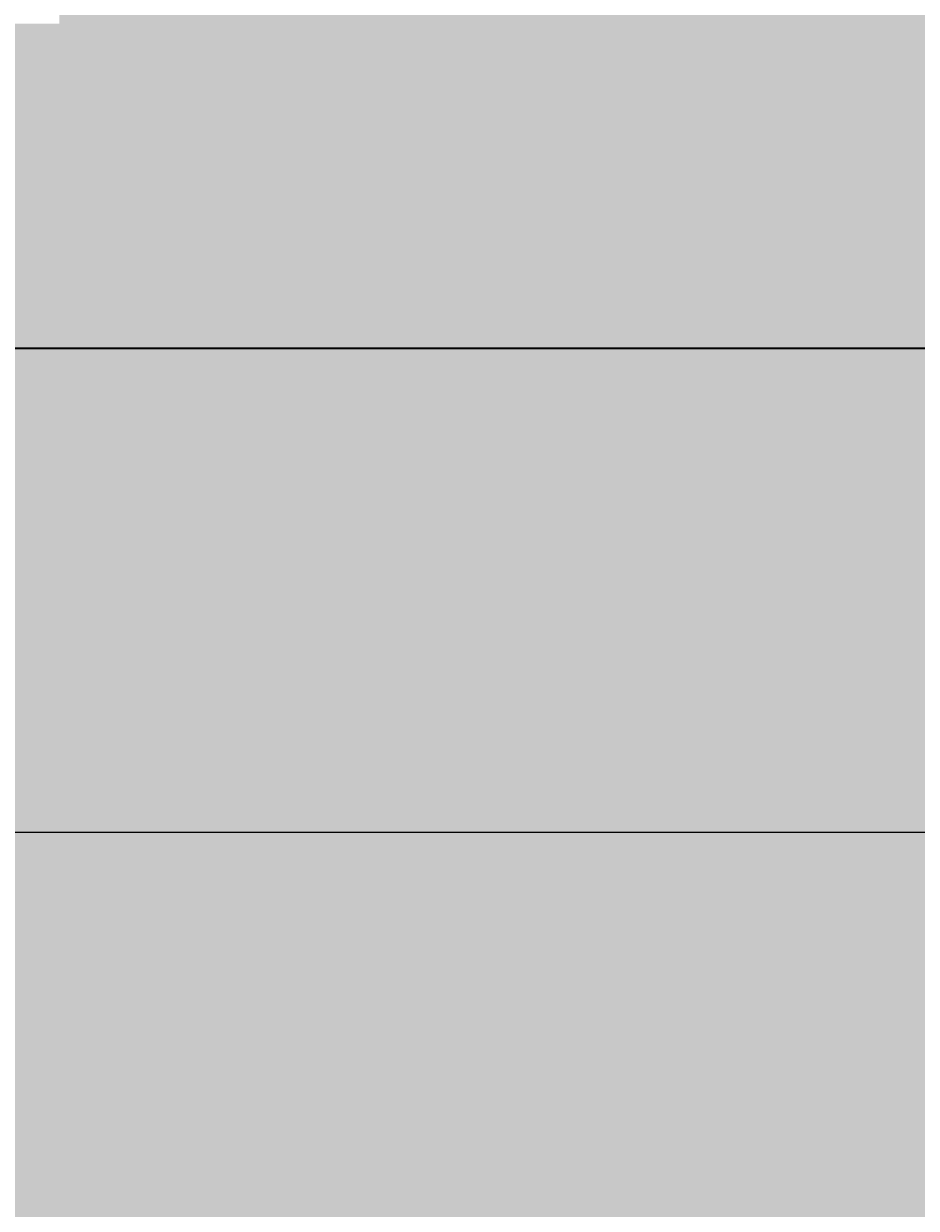
# Model space of a CAD drawing. Units: feet. Extents: x 2695 to 2912, y 795 to 1139.
# Tile 32 of 83: x 2842 to 2877, y 891 to 937. Entities that reach past the tile are written whole.
import ezdxf

# ---------------------------------------------------------------- set-up
doc = ezdxf.new("R2010")
doc.units = ezdxf.units.FT
for name, color, linetype, lineweight in [('A-ANNO-DIMS', 2, 'Continuous', 18), ('A-ELEV', 7, 'Continuous', 35), ('A-ELEV-PATT', 252, 'Continuous', 13)]:
    doc.layers.add(name, color=color, linetype=linetype, lineweight=lineweight)
doc.styles.get("Standard").update_dxf_attribs({"font": 'arial.ttf'})
doc.dimstyles.get("Standard").update_dxf_attribs({"dimtxt": 0.18, "dimasz": 0.18, "dimexe": 0.18, "dimexo": 0.0625, "dimgap": 0.09, "dimtad": 0, "dimtih": 1, "dimtoh": 1, "dimdec": 1, "dimzin": 0, "dimdsep": 46, "dimlunit": 3, "dimtxsty": 'Standard', "dimcen": 0.09, "dimadec": 0, "dimazin": 0, "dimtfac": 1, "dimtdec": 1, "dimtofl": 0, "dimtmove": 0, "dimatfit": 3, "dimfxl": 1, "dimtolj": 1, "dimtzin": 0, "dimarcsym": 0})

# ---------------------------------------------------------------- blocks, each defined once
blk = doc.blocks.new('*D14')
at = {"layer": 'A-ANNO-DIMS', "color": 0, "lineweight": -2, "transparency": 16777216}
for p, q in [((2838.439, 905.514), (2911.424, 905.514)), ((2911.244, 905.334), (2911.244, 890.368)), ((2911.244, 875.037), (2911.244, 890.004)), ((2758.214, 874.857), (2911.424, 874.857))]:
    blk.add_line(p, q, dxfattribs=at)
at = {"layer": 'A-ANNO-DIMS', "color": 0, "transparency": 16777216}
for points in [[(2911.214, 905.334), (2911.274, 905.334), (2911.244, 905.514)], [(2911.214, 875.037), (2911.274, 875.037), (2911.244, 874.857)]]:
    blk.add_solid(points, dxfattribs=at)
at = {"layer": 'Defpoints', "color": 0, "transparency": 16777216}
for p in [(2838.377, 905.514), (2911.244, 905.514), (2758.151, 874.857)]:
    blk.add_point(p, dxfattribs=at)
at = {"layer": 'A-ANNO-DIMS', "color": 0, "transparency": 16777216, "insert": (2911.244, 890.186), "char_height": 0.18, "attachment_point": 5}
blk.add_mtext('\\A1;30.66', dxfattribs=at)
blk = doc.blocks.new('*D15')
at = {"layer": 'A-ANNO-DIMS', "color": 0, "lineweight": -2, "transparency": 16777216}
for p, q in [((2890.699, 924.311), (2911.424, 924.311)), ((2911.244, 924.131), (2911.244, 915.094)), ((2911.244, 905.694), (2911.244, 914.731)), ((2838.439, 905.514), (2911.424, 905.514))]:
    blk.add_line(p, q, dxfattribs=at)
at = {"layer": 'A-ANNO-DIMS', "color": 0, "transparency": 16777216}
for points in [[(2911.214, 924.131), (2911.274, 924.131), (2911.244, 924.311)], [(2911.214, 905.694), (2911.274, 905.694), (2911.244, 905.514)]]:
    blk.add_solid(points, dxfattribs=at)
at = {"layer": 'Defpoints', "color": 0, "transparency": 16777216}
for p in [(2890.636, 924.311), (2911.244, 924.311), (2838.377, 905.514)]:
    blk.add_point(p, dxfattribs=at)
at = {"layer": 'A-ANNO-DIMS', "color": 0, "transparency": 16777216, "insert": (2911.244, 914.912), "char_height": 0.18, "attachment_point": 5}
blk.add_mtext('\\A1;18.796', dxfattribs=at)
blk = doc.blocks.new('*D17')
at = {"layer": 'A-ANNO-DIMS', "color": 0, "lineweight": -2, "transparency": 16777216}
for p, q in [((2843.637, 1020.824), (2911.424, 1020.824)), ((2911.244, 1020.644), (2911.244, 979.059)), ((2911.244, 937.111), (2911.244, 978.695)), ((2890.699, 936.931), (2911.424, 936.931))]:
    blk.add_line(p, q, dxfattribs=at)
at = {"layer": 'A-ANNO-DIMS', "color": 0, "transparency": 16777216}
for points in [[(2911.214, 1020.644), (2911.274, 1020.644), (2911.244, 1020.824)], [(2911.214, 937.111), (2911.274, 937.111), (2911.244, 936.931)]]:
    blk.add_solid(points, dxfattribs=at)
at = {"layer": 'Defpoints', "color": 0, "transparency": 16777216}
for p in [(2843.575, 1020.824), (2911.244, 1020.824), (2890.636, 936.931)]:
    blk.add_point(p, dxfattribs=at)
at = {"layer": 'A-ANNO-DIMS', "color": 0, "transparency": 16777216, "insert": (2911.244, 978.877), "char_height": 0.18, "attachment_point": 5}
blk.add_mtext('\\A1;83.9', dxfattribs=at)

msp = doc.modelspace()

# ---------------------------------------------------------------- hatches: boundary and pattern name
at = {"layer": 'A-ELEV-PATT'}
h = msp.add_hatch(color=256, dxfattribs=at)
h.set_gradient(color1=(255, 255, 255), tint=1)
h.paths.add_polyline_path([(2770.6361, 1122.9306), (2710.6361, 1122.9306), (2710.6361, 1118.4096), (2770.6361, 1118.4096)])
h.paths.add_polyline_path([(2890.6361, 1107.8588), (2770.6361, 1107.8588), (2770.6361, 1103.3378), (2890.6361, 1103.3378)])
h.paths.add_polyline_path([(2890.6361, 1062.9306), (2710.6361, 1062.9306), (2710.6361, 1056.9306), (2710.6361, 936.9306), (2710.6361, 924.3105), (2716.5358, 924.3105), (2890.6361, 924.3105), (2890.6361, 936.9306), (2715.8852, 936.9306), (2715.8852, 1050.3105), (2890.6361, 1050.3105)])
h.paths.add_polyline_path([(2716.5358, 924.3105), (2710.6361, 924.3105), (2710.6361, 810.9306), (2716.5358, 810.9306)])
h = msp.add_hatch(color=256, dxfattribs=at)
h.set_gradient(color1=(147, 149, 152), color2=(147, 149, 152), tint=1)
h.paths.add_polyline_path([(2770.6361, 1118.4096), (2710.6361, 1118.4096), (2710.6361, 1062.9306), (2770.6361, 1062.9306)])
h.paths.add_polyline_path([(2890.6361, 1103.3378), (2770.6361, 1103.3378), (2770.6361, 1062.9306), (2890.6361, 1062.9306)])
h.paths.add_polyline_path([(2730.7081, 1048.1052), (2755.1125, 1048.1052), (2755.1125, 936.9306), (2770.6361, 936.9306), (2770.6361, 1050.3105), (2715.8852, 1050.3105), (2715.8852, 936.9306), (2730.7081, 936.9306)])
h.paths.add_polyline_path([(2890.6361, 1050.3105), (2770.6361, 1050.3105), (2770.6361, 971.9673), (2778.0341, 971.9673), (2778.0341, 1020.8235), (2843.575, 1020.8235), (2843.575, 971.9673), (2890.6361, 971.9673)])
h.paths.add_polyline_path([(2888.1882, 970.7156), (2843.575, 970.7156), (2843.575, 964.8267), (2888.1882, 964.8267)])
h.paths.add_polyline_path([(2888.1882, 964.1328), (2843.575, 964.1328), (2843.575, 956.614), (2888.1882, 956.614)])
h.paths.add_polyline_path([(2888.1882, 955.9202), (2843.575, 955.9202), (2843.575, 949.2892), (2888.1882, 949.2892)])
h.paths.add_polyline_path([(2888.1882, 948.5954), (2843.575, 948.5954), (2843.575, 941.3507), (2888.1882, 941.3507)])
h.paths.add_polyline_path([(2888.1882, 940.6569), (2843.575, 940.6569), (2843.575, 936.9306), (2888.1882, 936.9306)])
h.paths.add_polyline_path([(2890.6361, 970.7156), (2888.9368, 970.7156), (2888.9368, 964.8267), (2890.6361, 964.8267)])
h.paths.add_polyline_path([(2890.6361, 964.1328), (2888.9368, 964.1328), (2888.9368, 956.614), (2890.6361, 956.614)])
h.paths.add_polyline_path([(2890.6361, 955.9202), (2888.9368, 955.9202), (2888.9368, 949.2892), (2890.6361, 949.2892)])
h.paths.add_polyline_path([(2890.6361, 940.6569), (2888.9368, 940.6569), (2888.9368, 936.9306), (2890.6361, 936.9306)])
h.paths.add_polyline_path([(2890.6361, 948.5954), (2888.9368, 948.5954), (2888.9368, 941.3507), (2890.6361, 941.3507)])
h.paths.add_polyline_path([(2772.5216, 970.7156), (2770.6361, 970.7156), (2770.6361, 964.8267), (2772.5216, 964.8267)])
h.paths.add_polyline_path([(2772.5216, 964.1328), (2770.6361, 964.1328), (2770.6361, 956.614), (2772.5216, 956.614)])
h.paths.add_polyline_path([(2772.5216, 955.9202), (2770.6361, 955.9202), (2770.6361, 949.2892), (2772.5216, 949.2892)])
h.paths.add_polyline_path([(2772.5216, 948.5954), (2770.6361, 948.5954), (2770.6361, 941.3507), (2772.5216, 941.3507)])
h.paths.add_polyline_path([(2772.5216, 940.6569), (2770.6361, 940.6569), (2770.6361, 936.9306), (2772.5216, 936.9306)])
h.paths.add_polyline_path([(2778.0341, 940.6569), (2773.2702, 940.6569), (2773.2702, 936.9306), (2778.0341, 936.9306)])
h.paths.add_polyline_path([(2778.0341, 970.7156), (2773.2702, 970.7156), (2773.2702, 964.8267), (2778.0341, 964.8267)])
h.paths.add_polyline_path([(2778.0341, 964.1328), (2773.2702, 964.1328), (2773.2702, 956.614), (2778.0341, 956.614)])
h.paths.add_polyline_path([(2778.0341, 955.9202), (2773.2702, 955.9202), (2773.2702, 949.2892), (2778.0341, 949.2892)])
h.paths.add_polyline_path([(2778.0341, 948.5954), (2773.2702, 948.5954), (2773.2702, 941.3507), (2778.0341, 941.3507)])
h.paths.add_polyline_path([(2810.0407, 940.6569), (2780.0341, 940.6569), (2780.0341, 936.9306), (2810.0407, 936.9306)])
h.paths.add_polyline_path([(2890.6361, 924.3105), (2770.6361, 924.3105), (2770.6361, 810.9306), (2773.5029, 810.9306), (2773.5029, 905.5143), (2805.9398, 905.5143), (2838.3767, 905.5143), (2838.3767, 810.9306), (2890.6361, 810.9306)])

# ---------------------------------------------------------------- linework, layer by layer
at = {"layer": 'A-ELEV'}
msp.add_lwpolyline([(2890.6361, 936.9306), (2890.6361, 924.3105), (2710.6361, 924.3105), (2710.6361, 936.9306)], dxfattribs=at)

# ---------------------------------------------------------------- dimensions: what is measured, and where the dimension line sits
at = {"layer": 'A-ANNO-DIMS'}
for base, p1, p2, override, picture, middle in [((2911.2444, 1020.8235), (2890.6361, 936.9306), (2843.575, 1020.8235), {"dimdec": 1, "dimlfac": 1, "dimrnd": 0, "dimzin": 0, "dimdsep": 46, "dimlunit": 2}, '*D17', (2911.2444, 978.877)), ((2911.2444, 924.3105), (2838.3767, 905.5143), (2890.6361, 924.3105), {"dimdec": 3, "dimlfac": 1, "dimrnd": 0, "dimzin": 0, "dimdsep": 46, "dimlunit": 2}, '*D15', (2911.2444, 914.9124)), ((2911.2444, 905.5143), (2758.1515, 874.8571), (2838.3767, 905.5143), {"dimdec": 2, "dimlfac": 1, "dimrnd": 0, "dimzin": 0, "dimdsep": 46, "dimlunit": 2}, '*D14', (2911.2444, 890.1857))]:
    dim = msp.add_linear_dim(base=base, p1=p1, p2=p2, angle=90, dimstyle='Standard', override=override, dxfattribs=at)
    dim.commit()
    dim.dimension.update_dxf_attribs({"geometry": picture, "text_midpoint": middle})

doc.saveas('drawing.dxf')
